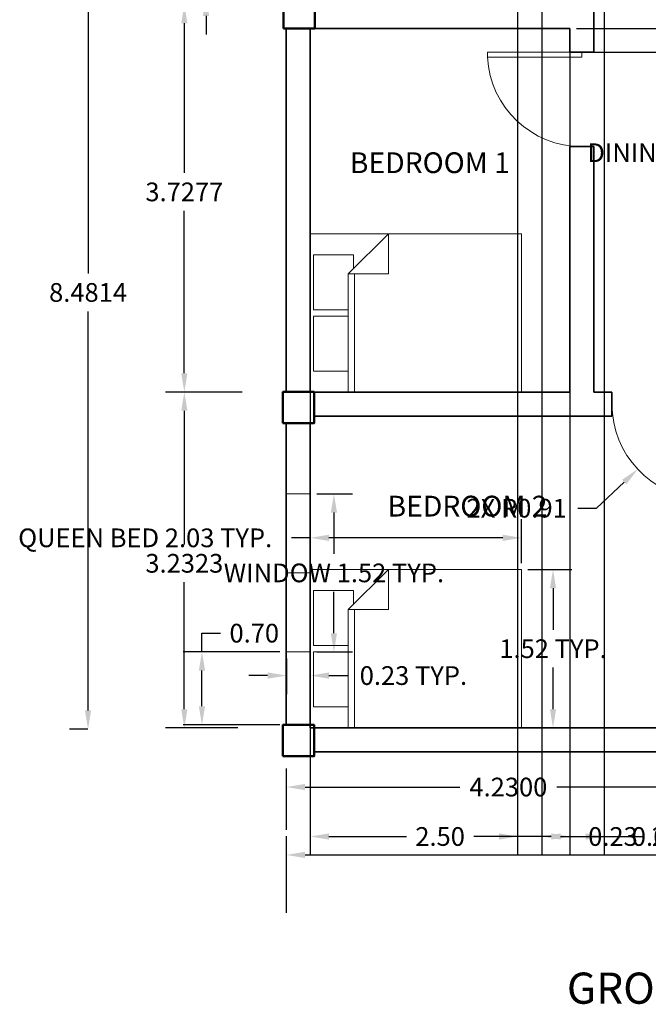
# Model space of a CAD drawing. Units: metres. Extents: x 473.2 to 488.6, y 701.8 to 717.3.
# Tile 1 of 4: x 473.2 to 479.3, y 701.8 to 711.3. Entities that reach past the tile are written whole.
import ezdxf

# ---------------------------------------------------------------- set-up
doc = ezdxf.new("R2010")
doc.units = ezdxf.units.M
doc.header["$PDMODE"] = 32
for name, color, linetype, lineweight in [('A-ANNO-DIMS', 2, 'Continuous', 18), ('A-ANNO-TEXT', 7, 'Continuous', 25), ('A-AREA-IDEN', 7, 'Continuous', 18), ('A-COLS', 7, 'Continuous', 50), ('A-DOOR', 3, 'Continuous', 18), ('A-FURN', 8, 'Continuous', 18), ('A-GLAZ', 4, 'Continuous', 18), ('A-WALL', 7, 'Continuous', 35)]:
    doc.layers.add(name, color=color, linetype=linetype, lineweight=lineweight)
doc.styles.get("Standard").update_dxf_attribs({"font": 'arial.ttf'})
doc.dimstyles.get("Standard").update_dxf_attribs({"dimtxt": 0.18, "dimasz": 0.18, "dimexe": 0.18, "dimexo": 0.0625, "dimgap": 0.09, "dimtad": 0, "dimtih": 1, "dimtoh": 1, "dimdec": 4, "dimzin": 0, "dimdsep": 46, "dimtxsty": 'Standard', "dimcen": 0.09, "dimadec": 0, "dimazin": 0, "dimtfac": 1, "dimtdec": 4, "dimtofl": 0, "dimtmove": 0, "dimatfit": 3, "dimfxl": 1, "dimtolj": 1, "dimtzin": 0, "dimarcsym": 0})

# ---------------------------------------------------------------- blocks, each defined once
blk = doc.blocks.new('Bed - Queen')
for p, q in [((0, -80.00003), (0, 0)), ((0, 0), (59.99999, 0)), ((59.99999, 0), (59.99999, -80.00003)), ((7.99999, -1.2), (28.79998, -1.2)), ((7.99999, -14.4), (7.99999, -1.2)), ((28.79998, -1.2), (28.79998, -14.4)), ((31.19999, -1.2), (51.99999, -1.2)), ((31.19999, -14.4), (31.19999, -1.2)), ((51.99999, -1.2), (51.99999, -16.4)), ((0, -14.4), (44.8, -14.4)), ((59.99999, -29.6), (44.8, -14.4)), ((44.8, -14.4), (44.8, -29.6)), ((44.8, -16.8), (0, -16.8)), ((51.99999, -16.4), (46.79936, -16.4)), ((44.8, -29.6), (59.99999, -29.6)), ((59.99999, -80.00003), (0, -80.00003))]:
    blk.add_line(p, q)
blk = doc.blocks.new('*D11')
at = {"layer": 'A-ANNO-DIMS', "color": 0, "lineweight": -2, "transparency": 16777216}
for p, q in [((475.0815, 711.4046), (474.6363, 711.4046)), ((474.8163, 711.2246), (474.8163, 709.7844)), ((474.8163, 707.8568), (474.8163, 709.4205)), ((475.3729, 707.6768), (474.6363, 707.6768))]:
    blk.add_line(p, q, dxfattribs=at)
at = {"layer": 'A-ANNO-DIMS', "color": 0, "transparency": 16777216}
for points in [[(474.7863, 711.2246), (474.8463, 711.2246), (474.8163, 711.4046)], [(474.7863, 707.8568), (474.8463, 707.8568), (474.8163, 707.6768)]]:
    blk.add_solid(points, dxfattribs=at)
at = {"layer": 'Defpoints', "color": 0, "transparency": 16777216}
for p in [(474.8163, 711.4046), (475.144, 711.4046), (475.4354, 707.6768)]:
    blk.add_point(p, dxfattribs=at)
at = {"layer": 'A-ANNO-DIMS', "color": 0, "transparency": 16777216, "insert": (474.8163, 709.6025), "char_height": 0.18, "width": 1.240263, "attachment_point": 5}
blk.add_mtext('\\A1;3.7277', dxfattribs=at)
blk = doc.blocks.new('*D12')
at = {"layer": 'A-ANNO-DIMS', "color": 0, "lineweight": -2, "transparency": 16777216}
for p, q in [((475.0389, 707.6768), (474.6363, 707.6768)), ((474.8163, 707.4968), (474.8163, 706.2104)), ((474.8163, 704.6246), (474.8163, 705.8465)), ((475.3303, 704.4446), (474.6363, 704.4446))]:
    blk.add_line(p, q, dxfattribs=at)
at = {"layer": 'A-ANNO-DIMS', "color": 0, "transparency": 16777216}
for points in [[(474.7863, 707.4968), (474.8463, 707.4968), (474.8163, 707.6768)], [(474.7863, 704.6246), (474.8463, 704.6246), (474.8163, 704.4446)]]:
    blk.add_solid(points, dxfattribs=at)
at = {"layer": 'Defpoints', "color": 0, "transparency": 16777216}
for p in [(474.8163, 707.6768), (475.1014, 707.6768), (475.3928, 704.4446)]:
    blk.add_point(p, dxfattribs=at)
at = {"layer": 'A-ANNO-DIMS', "color": 0, "transparency": 16777216, "insert": (474.8163, 706.0285), "char_height": 0.18, "width": 1.240263, "attachment_point": 5}
blk.add_mtext('\\A1;3.2323', dxfattribs=at)
blk = doc.blocks.new('*D13')
at = {"layer": 'A-ANNO-DIMS', "color": 0, "lineweight": -2, "transparency": 16777216}
for p, q in [((474.139, 712.9138), (473.7097, 712.9138)), ((473.8897, 712.7338), (473.8897, 708.8168)), ((473.8897, 704.6124), (473.8897, 708.4529)), ((473.8891, 704.4324), (473.7097, 704.4324))]:
    blk.add_line(p, q, dxfattribs=at)
at = {"layer": 'A-ANNO-DIMS', "color": 0, "transparency": 16777216}
for points in [[(473.8597, 712.7338), (473.9197, 712.7338), (473.8897, 712.9138)], [(473.8597, 704.6124), (473.9197, 704.6124), (473.8897, 704.4324)]]:
    blk.add_solid(points, dxfattribs=at)
at = {"layer": 'Defpoints', "color": 0, "transparency": 16777216}
for p in [(473.8897, 712.9138), (474.2015, 712.9138), (473.9516, 704.4324)]:
    blk.add_point(p, dxfattribs=at)
at = {"layer": 'A-ANNO-DIMS', "color": 0, "transparency": 16777216, "insert": (473.8897, 708.6349), "char_height": 0.18, "width": 1.240263, "attachment_point": 5}
blk.add_mtext('\\A1;8.4814', dxfattribs=at)
blk = doc.blocks.new('*D18')
at = {"layer": 'A-ANNO-DIMS', "color": 0, "lineweight": -2, "transparency": 16777216}
for p, q in [((475.798, 702.6656), (475.798, 703.4022)), ((485.74, 702.957), (485.74, 703.4022)), ((475.978, 703.2222), (480.3782, 703.2222)), ((485.56, 703.2222), (481.3049, 703.2222))]:
    blk.add_line(p, q, dxfattribs=at)
at = {"layer": 'A-ANNO-DIMS', "color": 0, "transparency": 16777216}
for points in [[(475.978, 703.2522), (475.978, 703.1922), (475.798, 703.2222)], [(485.56, 703.2522), (485.56, 703.1922), (485.74, 703.2222)]]:
    blk.add_solid(points, dxfattribs=at)
at = {"layer": 'Defpoints', "color": 0, "transparency": 16777216}
for p in [(485.74, 703.2222), (485.74, 702.8945), (475.798, 702.6031)]:
    blk.add_point(p, dxfattribs=at)
at = {"layer": 'A-ANNO-DIMS', "color": 0, "transparency": 16777216, "insert": (480.8416, 703.2222), "char_height": 0.18, "width": 1.240263, "attachment_point": 5}
blk.add_mtext('\\A1;9.9420', dxfattribs=at)
blk = doc.blocks.new('*D19')
at = {"layer": 'A-ANNO-DIMS', "color": 0, "lineweight": -2, "transparency": 16777216}
for p, q in [((475.798, 703.4647), (475.798, 704.0553)), ((480.028, 703.6173), (480.028, 704.0553)), ((475.978, 703.8753), (477.468, 703.8753)), ((479.848, 703.8753), (478.4019, 703.8753))]:
    blk.add_line(p, q, dxfattribs=at)
at = {"layer": 'A-ANNO-DIMS', "color": 0, "transparency": 16777216}
for points in [[(475.978, 703.9053), (475.978, 703.8453), (475.798, 703.8753)], [(479.848, 703.9053), (479.848, 703.8453), (480.028, 703.8753)]]:
    blk.add_solid(points, dxfattribs=at)
at = {"layer": 'Defpoints', "color": 0, "transparency": 16777216}
for p in [(480.028, 703.8753), (480.028, 703.5548), (475.798, 703.4022)]:
    blk.add_point(p, dxfattribs=at)
at = {"layer": 'A-ANNO-DIMS', "color": 0, "transparency": 16777216, "insert": (477.9349, 703.8753), "char_height": 0.18, "width": 1.240263, "attachment_point": 5}
blk.add_mtext('\\A1;4.2300', dxfattribs=at)
blk = doc.blocks.new('DOOR-SWING-910')
for p, q in [((0, 0), (-0.05, 0)), ((-0.05, 0), (-0.05, -0.91)), ((0, 0), (0, -0.91)), ((0, -0.91), (-0.05, -0.91))]:
    blk.add_line(p, q)
blk.add_arc((0.0015, 0), 0.9115, 180, 266.76381)
blk = doc.blocks.new('COL-SQUARE-300')
blk.add_lwpolyline([(-0.15, -0.15), (0.15, -0.15), (0.15, 0.15), (-0.15, 0.15)], close=True)
blk = doc.blocks.new('WIN-1520')
blk.add_line((0.23, 0.76), (0, 0.76))
blk.add_lwpolyline([(0.23, 0), (0.23, 1.52), (0, 1.52), (0, 0)], close=True)
blk = doc.blocks.new('*D29')
at = {"layer": 'A-ANNO-DIMS', "color": 0, "lineweight": -2, "transparency": 16777216}
for p, q in [((476.0905, 706.6961), (476.436, 706.6961)), ((476.256, 706.5161), (476.256, 706.1193)), ((476.256, 705.3561), (476.256, 705.753)), ((476.0905, 705.1761), (476.436, 705.1761))]:
    blk.add_line(p, q, dxfattribs=at)
at = {"layer": 'A-ANNO-DIMS', "color": 0, "transparency": 16777216}
for points in [[(476.226, 706.5161), (476.286, 706.5161), (476.256, 706.6961)], [(476.226, 705.3561), (476.286, 705.3561), (476.256, 705.1761)]]:
    blk.add_solid(points, dxfattribs=at)
at = {"layer": 'Defpoints', "color": 0, "transparency": 16777216}
for p in [(476.028, 706.6961), (476.256, 706.6961), (476.028, 705.1761)]:
    blk.add_point(p, dxfattribs=at)
at = {"layer": 'A-ANNO-DIMS', "color": 0, "transparency": 16777216, "insert": (476.256, 705.9361), "char_height": 0.18, "attachment_point": 5}
blk.add_mtext('\\A1;WINDOW 1.52 TYP.', dxfattribs=at)
blk = doc.blocks.new('*D30')
at = {"layer": 'A-ANNO-DIMS', "color": 0, "lineweight": -2, "transparency": 16777216}
for p, q in [((475.798, 705.1136), (475.798, 704.7681)), ((476.028, 705.1136), (476.028, 704.7681)), ((475.618, 704.9481), (475.438, 704.9481)), ((476.208, 704.9481), (476.388, 704.9481))]:
    blk.add_line(p, q, dxfattribs=at)
at = {"layer": 'A-ANNO-DIMS', "color": 0, "transparency": 16777216}
for points in [[(475.618, 704.9781), (475.618, 704.9181), (475.798, 704.9481)], [(476.208, 704.9781), (476.208, 704.9181), (476.028, 704.9481)]]:
    blk.add_solid(points, dxfattribs=at)
at = {"layer": 'Defpoints', "color": 0, "transparency": 16777216}
for p in [(475.798, 705.1761), (476.028, 705.1761), (476.028, 704.9481)]:
    blk.add_point(p, dxfattribs=at)
at = {"layer": 'A-ANNO-DIMS', "color": 0, "transparency": 16777216, "insert": (477.0209, 704.9481), "char_height": 0.18, "attachment_point": 5}
blk.add_mtext('\\A1;0.23 TYP.', dxfattribs=at)
blk = doc.blocks.new('*D31')
at = {"layer": 'A-ANNO-DIMS', "color": 0, "lineweight": -2, "transparency": 16777216}
for p, q in [((476.028, 706.0311), (476.028, 706.4534)), ((478.06, 706.0311), (478.06, 706.4534)), ((476.028, 706.2734), (475.848, 706.2734)), ((477.88, 706.2734), (476.208, 706.2734))]:
    blk.add_line(p, q, dxfattribs=at)
at = {"layer": 'A-ANNO-DIMS', "color": 0, "transparency": 16777216}
for points in [[(476.208, 706.3034), (476.208, 706.2434), (476.028, 706.2734)], [(477.88, 706.3034), (477.88, 706.2434), (478.06, 706.2734)]]:
    blk.add_solid(points, dxfattribs=at)
at = {"layer": 'Defpoints', "color": 0, "transparency": 16777216}
for p in [(476.028, 706.2734), (476.028, 705.9686), (478.06, 705.9686)]:
    blk.add_point(p, dxfattribs=at)
at = {"layer": 'A-ANNO-DIMS', "color": 0, "transparency": 16777216, "insert": (474.4397, 706.2734), "char_height": 0.18, "attachment_point": 5}
blk.add_mtext('\\A1;QUEEN BED 2.03 TYP.', dxfattribs=at)
blk = doc.blocks.new('*D32')
at = {"layer": 'A-ANNO-DIMS', "color": 0, "lineweight": -2, "transparency": 16777216}
for p, q in [((478.1225, 705.9686), (478.5448, 705.9686)), ((478.3648, 705.7886), (478.3648, 705.3885)), ((478.3648, 704.6246), (478.3648, 705.0247)), ((478.1225, 704.4446), (478.5448, 704.4446))]:
    blk.add_line(p, q, dxfattribs=at)
at = {"layer": 'A-ANNO-DIMS', "color": 0, "transparency": 16777216}
for points in [[(478.3348, 705.7886), (478.3948, 705.7886), (478.3648, 705.9686)], [(478.3348, 704.6246), (478.3948, 704.6246), (478.3648, 704.4446)]]:
    blk.add_solid(points, dxfattribs=at)
at = {"layer": 'Defpoints', "color": 0, "transparency": 16777216}
for p in [(478.06, 705.9686), (478.3648, 705.9686), (478.06, 704.4446)]:
    blk.add_point(p, dxfattribs=at)
at = {"layer": 'A-ANNO-DIMS', "color": 0, "transparency": 16777216, "insert": (478.3648, 705.2066), "char_height": 0.18, "attachment_point": 5}
blk.add_mtext('\\A1;1.52 TYP.', dxfattribs=at)
blk = doc.blocks.new('*D37')
at = {"layer": 'A-ANNO-DIMS', "color": 0, "lineweight": -2, "transparency": 16777216}
for p, q in [((479.9098, 711.1348), (479.4456, 711.1348)), ((479.6256, 710.9548), (479.6256, 710.1622)), ((479.6256, 709.0034), (479.6256, 709.796)), ((479.9098, 708.8234), (479.4456, 708.8234))]:
    blk.add_line(p, q, dxfattribs=at)
at = {"layer": 'A-ANNO-DIMS', "color": 0, "transparency": 16777216}
for points in [[(479.5956, 710.9548), (479.6556, 710.9548), (479.6256, 711.1348)], [(479.5956, 709.0034), (479.6556, 709.0034), (479.6256, 708.8234)]]:
    blk.add_solid(points, dxfattribs=at)
at = {"layer": 'Defpoints', "color": 0, "transparency": 16777216}
for p in [(479.9723, 711.1348), (479.6256, 708.8234), (479.9723, 708.8234)]:
    blk.add_point(p, dxfattribs=at)
at = {"layer": 'A-ANNO-DIMS', "color": 0, "transparency": 16777216, "insert": (479.6256, 709.9791), "char_height": 0.18, "attachment_point": 5}
blk.add_mtext('\\A1;DINING SET 2.31', dxfattribs=at)
blk = doc.blocks.new('*D43')
at = {"layer": 'A-ANNO-DIMS', "color": 0, "lineweight": -2, "transparency": 16777216}
for p, q in [((476.028, 711.1121), (476.028, 703.2195)), ((478.528, 711.1121), (478.528, 703.2195)), ((476.208, 703.3995), (476.953, 703.3995)), ((478.348, 703.3995), (477.603, 703.3995))]:
    blk.add_line(p, q, dxfattribs=at)
at = {"layer": 'A-ANNO-DIMS', "color": 0, "transparency": 16777216}
for points in [[(476.208, 703.4295), (476.208, 703.3695), (476.028, 703.3995)], [(478.348, 703.4295), (478.348, 703.3695), (478.528, 703.3995)]]:
    blk.add_solid(points, dxfattribs=at)
at = {"layer": 'Defpoints', "color": 0, "transparency": 16777216}
for p in [(476.028, 711.1746), (478.528, 711.1746), (478.528, 703.3995)]:
    blk.add_point(p, dxfattribs=at)
at = {"layer": 'A-ANNO-DIMS', "color": 0, "transparency": 16777216, "insert": (477.278, 703.3995), "char_height": 0.18, "attachment_point": 5}
blk.add_mtext('\\A1;2.50', dxfattribs=at)
blk = doc.blocks.new('*D44')
at = {"layer": 'A-ANNO-DIMS', "color": 0, "lineweight": -2, "transparency": 16777216}
for p, q in [((486.5158, 711.3546), (486.5158, 711.5346)), ((486.5158, 711.5346), (486.6958, 711.5346)), ((478.5905, 711.1746), (486.6958, 711.1746)), ((478.5905, 710.9478), (486.6958, 710.9478)), ((486.5158, 710.7678), (486.5158, 710.5878))]:
    blk.add_line(p, q, dxfattribs=at)
at = {"layer": 'A-ANNO-DIMS', "color": 0, "transparency": 16777216}
for points in [[(486.4858, 711.3546), (486.5458, 711.3546), (486.5158, 711.1746)], [(486.4858, 710.7678), (486.5458, 710.7678), (486.5158, 710.9478)]]:
    blk.add_solid(points, dxfattribs=at)
at = {"layer": 'Defpoints', "color": 0, "transparency": 16777216}
for p in [(478.528, 711.1746), (486.5158, 711.1746), (478.528, 710.9478)]:
    blk.add_point(p, dxfattribs=at)
at = {"layer": 'A-ANNO-DIMS', "color": 0, "transparency": 16777216, "insert": (487.0196, 711.5346), "char_height": 0.18, "attachment_point": 5}
blk.add_mtext('\\A1;0.23', dxfattribs=at)
blk = doc.blocks.new('*D54')
at = {"layer": 'A-ANNO-DIMS', "color": 0, "lineweight": -2, "transparency": 16777216}
for p, q in [((478.0241, 714.2595), (478.0241, 703.2195)), ((478.258, 714.2595), (478.258, 703.2195)), ((477.8441, 703.3995), (477.6641, 703.3995)), ((478.438, 703.3995), (478.618, 703.3995))]:
    blk.add_line(p, q, dxfattribs=at)
at = {"layer": 'A-ANNO-DIMS', "color": 0, "transparency": 16777216}
for points in [[(477.8441, 703.4295), (477.8441, 703.3695), (478.0241, 703.3995)], [(478.438, 703.4295), (478.438, 703.3695), (478.258, 703.3995)]]:
    blk.add_solid(points, dxfattribs=at)
at = {"layer": 'Defpoints', "color": 0, "transparency": 16777216}
for p in [(478.0241, 714.322), (478.258, 714.322), (478.258, 703.3995)]:
    blk.add_point(p, dxfattribs=at)
at = {"layer": 'A-ANNO-DIMS', "color": 0, "transparency": 16777216, "insert": (478.9417, 703.3995), "char_height": 0.18, "attachment_point": 5}
blk.add_mtext('\\A1;0.23', dxfattribs=at)
blk = doc.blocks.new('*D55')
at = {"layer": 'A-ANNO-DIMS', "color": 0, "lineweight": -2, "transparency": 16777216}
for p, q in [((474.9859, 705.1761), (474.9859, 705.3561)), ((474.9859, 705.3561), (475.1659, 705.3561)), ((475.7355, 705.1761), (474.8059, 705.1761)), ((474.9859, 704.6525), (474.9859, 704.9961)), ((475.7355, 704.4725), (474.8059, 704.4725))]:
    blk.add_line(p, q, dxfattribs=at)
at = {"layer": 'A-ANNO-DIMS', "color": 0, "transparency": 16777216}
for points in [[(474.9559, 704.9961), (475.0159, 704.9961), (474.9859, 705.1761)], [(474.9559, 704.6525), (475.0159, 704.6525), (474.9859, 704.4725)]]:
    blk.add_solid(points, dxfattribs=at)
at = {"layer": 'Defpoints', "color": 0, "transparency": 16777216}
for p in [(474.9859, 705.1761), (475.798, 705.1761), (475.798, 704.4725)]:
    blk.add_point(p, dxfattribs=at)
at = {"layer": 'A-ANNO-DIMS', "color": 0, "transparency": 16777216, "insert": (475.4893, 705.3561), "char_height": 0.18, "attachment_point": 5}
blk.add_mtext('\\A1;0.70', dxfattribs=at)
blk = doc.blocks.new('*D60')
at = {"layer": 'A-ANNO-DIMS', "color": 0, "lineweight": -2, "transparency": 16777216}
for p, q in [((475.025, 712.0601), (475.025, 712.2401)), ((475.7355, 711.8801), (474.845, 711.8801)), ((475.7355, 711.4754), (474.845, 711.4754)), ((475.025, 711.2954), (475.025, 711.1154))]:
    blk.add_line(p, q, dxfattribs=at)
at = {"layer": 'A-ANNO-DIMS', "color": 0, "transparency": 16777216}
for points in [[(474.995, 712.0601), (475.055, 712.0601), (475.025, 711.8801)], [(474.995, 711.2954), (475.055, 711.2954), (475.025, 711.4754)]]:
    blk.add_solid(points, dxfattribs=at)
at = {"layer": 'Defpoints', "color": 0, "transparency": 16777216}
for p in [(475.025, 711.8801), (475.798, 711.8801), (475.798, 711.4754)]:
    blk.add_point(p, dxfattribs=at)
at = {"layer": 'A-ANNO-DIMS', "color": 0, "transparency": 16777216, "insert": (475.025, 711.6777), "char_height": 0.18, "attachment_point": 5}
blk.add_mtext('\\A1;0.40', dxfattribs=at)
blk = doc.blocks.new('*D64')
at = {"layer": 'A-ANNO-DIMS', "color": 0, "lineweight": -2, "transparency": 16777216}
for p, q in [((478.258, 715.4721), (478.258, 703.2195)), ((480.8495, 715.4721), (480.8495, 703.2195)), ((478.438, 703.3995), (479.2283, 703.3995)), ((480.6695, 703.3995), (479.8793, 703.3995))]:
    blk.add_line(p, q, dxfattribs=at)
at = {"layer": 'A-ANNO-DIMS', "color": 0, "transparency": 16777216}
for points in [[(478.438, 703.4295), (478.438, 703.3695), (478.258, 703.3995)], [(480.6695, 703.4295), (480.6695, 703.3695), (480.8495, 703.3995)]]:
    blk.add_solid(points, dxfattribs=at)
at = {"layer": 'Defpoints', "color": 0, "transparency": 16777216}
for p in [(478.258, 715.5346), (480.8495, 715.5346), (480.8495, 703.3995)]:
    blk.add_point(p, dxfattribs=at)
at = {"layer": 'A-ANNO-DIMS', "color": 0, "transparency": 16777216, "insert": (479.5538, 703.3995), "char_height": 0.18, "attachment_point": 5}
blk.add_mtext('\\A1;2.59', dxfattribs=at)
blk = doc.blocks.new('*D66')
at = {"layer": 'A-ANNO-DIMS', "color": 0, "lineweight": -2, "transparency": 16777216}
for p, q in [((478.258, 714.9046), (478.258, 703.2195)), ((478.858, 714.9046), (478.858, 703.2195)), ((478.438, 703.3995), (478.678, 703.3995)), ((478.858, 703.3995), (479.038, 703.3995))]:
    blk.add_line(p, q, dxfattribs=at)
at = {"layer": 'A-ANNO-DIMS', "color": 0, "transparency": 16777216}
for points in [[(478.438, 703.4295), (478.438, 703.3695), (478.258, 703.3995)], [(478.678, 703.4295), (478.678, 703.3695), (478.858, 703.3995)]]:
    blk.add_solid(points, dxfattribs=at)
at = {"layer": 'Defpoints', "color": 0, "transparency": 16777216}
for p in [(478.258, 714.9671), (478.858, 714.9671), (478.858, 703.3995)]:
    blk.add_point(p, dxfattribs=at)
at = {"layer": 'A-ANNO-DIMS', "color": 0, "transparency": 16777216, "insert": (479.3614, 703.3995), "char_height": 0.18, "attachment_point": 5}
blk.add_mtext('\\A1;0.60', dxfattribs=at)
blk = doc.blocks.new('*D68')
at = {"layer": 'A-ANNO-DIMS', "color": 0, "lineweight": -2, "transparency": 16777216}
for p, q in [((479.8428, 707.4696), (479.8428, 707.6496)), ((479.7528, 707.5596), (479.9328, 707.5596)), ((478.7822, 706.5586), (479.049, 706.8104)), ((478.6022, 706.5586), (478.7822, 706.5586))]:
    blk.add_line(p, q, dxfattribs=at)
at = {"layer": 'A-ANNO-DIMS', "color": 0, "transparency": 16777216}
blk.add_solid([(479.0284, 706.8322), (479.0696, 706.7886), (479.1799, 706.9339)], dxfattribs=at)
at = {"layer": 'Defpoints', "color": 0, "transparency": 16777216}
for p in [(479.8428, 707.5596), (479.1799, 706.9339)]:
    blk.add_point(p, dxfattribs=at)
at = {"layer": 'A-ANNO-DIMS', "color": 0, "transparency": 16777216, "insert": (478.0148, 706.5586), "char_height": 0.18, "attachment_point": 5}
blk.add_mtext('\\A1;2X R0.91', dxfattribs=at)

msp = doc.modelspace()

# ---------------------------------------------------------------- linework, layer by layer
at = {"layer": 'A-GLAZ'}
for p, q in [((475.79797, 708.44198), (475.79797, 710.26198)), ((476.02797, 710.26198), (476.02797, 708.44198))]:
    msp.add_line(p, q, dxfattribs=at)
at = {"layer": 'A-WALL'}
for p, q in [((478.75797, 710.94776), (478.75797, 711.40456)), ((475.79797, 707.67682), (475.79797, 711.17539)), ((476.02797, 711.17456), (478.52797, 711.17456)), ((476.02797, 707.67456), (476.02797, 711.17456)), ((478.52797, 710.94776), (478.52797, 711.17456)), ((478.52797, 710.94776), (478.75797, 710.94776)), ((478.52797, 707.67456), (478.52797, 710.03776)), ((478.52797, 710.03776), (478.75797, 710.03776)), ((478.75797, 707.67456), (478.75797, 710.03776)), ((476.02797, 707.67456), (478.52797, 707.67456)), ((478.75797, 707.67456), (478.93132, 707.67456)), ((478.93132, 707.67456), (478.93132, 707.44456)), ((476.06472, 707.44456), (478.93132, 707.44456)), ((475.79797, 704.4725), (475.79797, 707.37682)), ((476.02797, 704.44456), (476.02797, 707.37682)), ((476.02797, 704.44456), (479.98215, 704.44456)), ((476.06459, 704.21456), (479.98215, 704.21456))]:
    msp.add_line(p, q, dxfattribs=at)

# ---------------------------------------------------------------- block references
at = {"layer": 'A-COLS'}
for p in [(475.92166, 711.32539), (475.91472, 707.52682), (475.91459, 704.3225)]:
    msp.add_blockref('COL-SQUARE-300', p, dxfattribs=at)
at = {"layer": 'A-DOOR', "extrusion": (0, 0, -1), "zscale": -1, "rotation": 89.9999999999969}
msp.add_blockref('DOOR-SWING-910', (-478.64297, 710.94776), dxfattribs=at)
at = {"layer": 'A-DOOR'}
msp.add_blockref('DOOR-SWING-910', (479.84132, 707.55956), dxfattribs=at)
at = {"layer": 'A-FURN', "xscale": 0.0254, "yscale": 0.0254, "zscale": 0.0254, "rotation": 90}
for p in [(476.02797, 707.67456), (476.02797, 704.44456)]:
    msp.add_blockref('Bed - Queen', p, dxfattribs=at)
at = {"layer": 'A-GLAZ'}
msp.add_blockref('WIN-1520', (475.79797, 705.17613), dxfattribs=at)

# ---------------------------------------------------------------- texts
at = {"layer": 'A-ANNO-TEXT', "insert": (478.49827, 702.09007), "char_height": 0.3, "attachment_point": 1}
msp.add_mtext_dynamic_manual_height_columns('GROUND FLOOR PLAN', width=7.0056545, gutter_width=12.5, heights=[0.69309], dxfattribs=at)
at = {"layer": 'A-AREA-IDEN', "char_height": 0.2, "attachment_point": 1}
for s, insert in [('BEDROOM 1', (476.40905, 709.98299)), ('BEDROOM 2', (476.77163, 706.67854))]:
    msp.add_mtext_dynamic_manual_height_columns(s, width=2.8211562, gutter_width=12.5, heights=[0], dxfattribs=dict(at, insert=insert))

# ---------------------------------------------------------------- dimensions: what is measured, and where the dimension line sits
at = {"layer": 'A-ANNO-DIMS'}
for base, p1, p2, picture, middle in [((480.84954, 703.3995), (478.25797, 715.53456), (480.84954, 715.53456), '*D64', (479.55376, 703.3995)), ((478.85797, 703.3995), (478.25797, 714.9671), (478.85797, 714.9671), '*D66', (479.36144, 703.3995)), ((478.25797, 703.3995), (478.02407, 714.32196), (478.25797, 714.32196), '*D54', (478.94175, 703.3995)), ((478.52797, 703.3995), (476.02797, 711.17456), (478.52797, 711.17456), '*D43', (477.27797, 703.3995))]:
    dim = msp.add_linear_dim(base=base, p1=p1, p2=p2, dimstyle='Standard', override={"dimdec": 2, "dimlfac": 1, "dimrnd": 0, "dimzin": 0, "dimdsep": 46, "dimlunit": 2}, dxfattribs=at)
    dim.commit()
    dim.dimension.update_dxf_attribs({"geometry": picture, "text_midpoint": middle})
for base, p1, p2, picture, middle in [((473.88966, 712.91383), (473.95159, 704.4324), (474.20147, 712.91383), '*D13', (473.88966, 708.63485)), ((474.81629, 711.40456), (475.43544, 707.67682), (475.14404, 711.40456), '*D11', (474.81629, 709.60247)), ((474.81629, 707.67682), (475.39281, 704.44456), (475.10142, 707.67682), '*D12', (474.81629, 706.02846))]:
    dim = msp.add_linear_dim(base=base, p1=p1, p2=p2, angle=90, dimstyle='Standard', override={"dimclrd": 0, "dimclre": 0, "dimclrt": 0}, dxfattribs=at)
    dim.commit()
    dim.dimension.update_dxf_attribs({"geometry": picture, "text_midpoint": middle, "dimtype": 160})
for base, p1, p2, picture, middle in [((475.02497, 711.88009), (475.79797, 711.47539), (475.79797, 711.88009), '*D60', (475.02497, 711.67774)), ((486.51584, 711.17456), (478.52797, 710.94776), (478.52797, 711.17456), '*D44', (487.01962, 711.53456)), ((474.98588, 705.17612), (475.79797, 704.4725), (475.79797, 705.17612), '*D55', (475.48935, 705.35612))]:
    dim = msp.add_linear_dim(base=base, p1=p1, p2=p2, angle=90, dimstyle='Standard', override={"dimdec": 2, "dimlfac": 1, "dimrnd": 0, "dimzin": 0, "dimdsep": 46, "dimlunit": 2}, dxfattribs=at)
    dim.commit()
    dim.dimension.update_dxf_attribs({"geometry": picture, "text_midpoint": middle})
for base, p1, p2, angle, text, picture, middle in [((479.62562, 708.82342), (479.97233, 711.13482), (479.97233, 708.82342), 270, 'DINING SET <>', '*D37', (479.62562, 709.97912)), ((476.02797, 706.27336), (478.05997, 705.96856), (476.02797, 705.96856), 180, 'QUEEN BED <> TYP.', '*D31', (474.43971, 706.27336)), ((476.25597, 706.69613), (476.02797, 705.17613), (476.02797, 706.69613), 90, 'WINDOW <> TYP.', '*D29', (476.25597, 705.93613)), ((478.36477, 705.96856), (478.05997, 704.44456), (478.05997, 705.96856), 90, '<> TYP.', '*D32', (478.36477, 705.20656))]:
    dim = msp.add_linear_dim(base=base, p1=p1, p2=p2, angle=angle, text=text, dimstyle='Standard', override={"dimdec": 2, "dimlfac": 1, "dimrnd": 0, "dimzin": 0, "dimdsep": 46, "dimlunit": 2}, dxfattribs=at)
    dim.commit()
    dim.dimension.update_dxf_attribs({"geometry": picture, "text_midpoint": middle})
dim = msp.add_radius_dim(center=(479.84277, 707.55956), mpoint=(479.17994, 706.93394), text='2X <>', dimstyle='Standard', override={"dimdec": 2, "dimlfac": 1, "dimrnd": 0, "dimzin": 0, "dimdsep": 46, "dimlunit": 2}, dxfattribs=at)
dim.commit()
dim.dimension.update_dxf_attribs({"geometry": '*D68', "text_midpoint": (478.01478, 706.55857), "dimtype": 164})
dim = msp.add_linear_dim(base=(476.02797, 704.94813), p1=(475.79797, 705.17613), p2=(476.02797, 705.17613), text='<> TYP.', dimstyle='Standard', override={"dimdec": 2, "dimlfac": 1, "dimrnd": 0, "dimzin": 0, "dimdsep": 46, "dimlunit": 2}, dxfattribs=at)
dim.commit()
dim.dimension.update_dxf_attribs({"geometry": '*D30', "text_midpoint": (477.02091, 704.94813)})
for base, p1, p2, picture, middle in [((480.02797, 703.87534), (475.79797, 703.40224), (480.02797, 703.55481), '*D19', (477.93495, 703.87534)), ((485.73996, 703.22224), (475.79797, 702.6031), (485.73996, 702.8945), '*D18', (480.84155, 703.22224))]:
    dim = msp.add_linear_dim(base=base, p1=p1, p2=p2, dimstyle='Standard', override={"dimclrd": 0, "dimclre": 0, "dimclrt": 0}, dxfattribs=at)
    dim.commit()
    dim.dimension.update_dxf_attribs({"geometry": picture, "text_midpoint": middle, "dimtype": 160})

doc.saveas('drawing.dxf')
